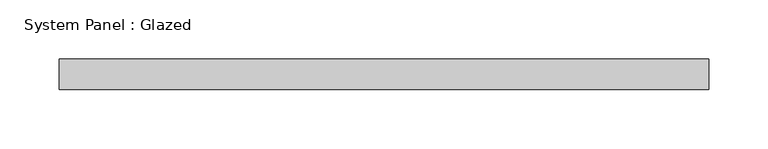
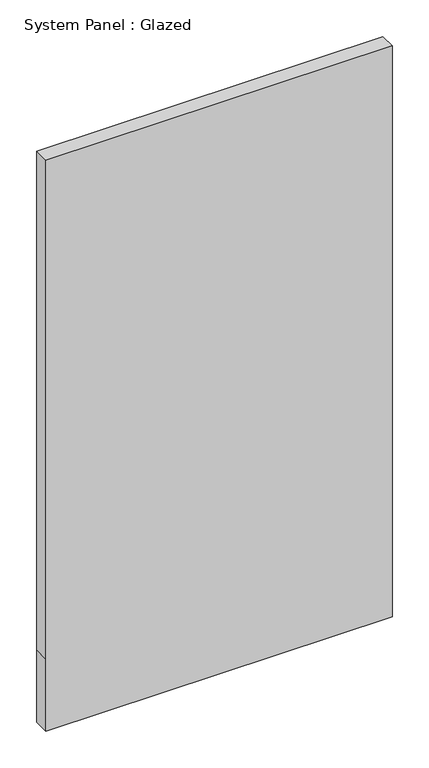
"""IFC4 building model written with IfcOpenShell, lengths in millimetres: plate geometry, System Panel : Glazed."""

from ifc_helpers import new_model, si_unit, frame, origin, place, context, project, spatial, polyline, outline, extrude, source, transform, mapped, element, save


def system_panel_glazed_51e75bbe(model_context):
    return source(origin(), model_context, "Body", "SweptSolid", [
        extrude(outline(polyline([(0.0, -273.05), (0.0, 273.05), (120.65, 273.05), (952.0990947, 273.05), (952.0990947, -273.05), (120.65, -273.05), (0.0, -273.05)])), frame((0.0, 19.05, 0.0), z_axis=(0.0, 1.0, 0.0), x_axis=(0.0, 0.0, 1.0)), (0.0, 0.0, 1.0), 25.4),
    ])


if __name__ == "__main__":
    model = new_model("IFC4")
    model_context = context("Model", 3, world=origin())
    ifc_project = project(units=[si_unit("LENGTHUNIT", "METRE", prefix="MILLI")], contexts=[model_context])
    site = spatial("IfcSite", under=ifc_project)
    building = spatial("IfcBuilding", under=site)
    placement = place(None, origin())
    system_panel_glazed_shape = system_panel_glazed_51e75bbe(model_context)
    element("IfcPlate", 1, ObjectType="System Panel : Glazed", at=placement, inside=building, context=model_context, shape_type="MappedRepresentation", body=[
        mapped(system_panel_glazed_shape, transform((0.0, 0.0, 0.0), x_axis=(1.0, 0.0, 0.0), y_axis=(0.0, 1.0, 0.0), z_axis=(0.0, 0.0, 1.0))),
    ])
    save(model, "model.ifc")

# Revit data of these elements
# Type "System Panel : Glazed"
#   Construction Type Id = "GSP4R"
#   Analytic Construction = "1/8 in Pilkington single glazing"
#   Visual Light Transmittance = 0.9
#   Solar Heat Gain Coefficient = 0.86
#   Heat Transfer Coefficient (U) = 1.18115 BTU/(h·ft²·°F)
#   Define Thermal Properties by = 1
# Element 1 (IfcPlate, "System Panel : Glazed")
#   Materials on its faces: "Glass"
# Materials
#   "Glass": class "Glass", colour RGB 0 128 192, transparency 0.75, Description = "Soda Lime Glass", Cost = 0
